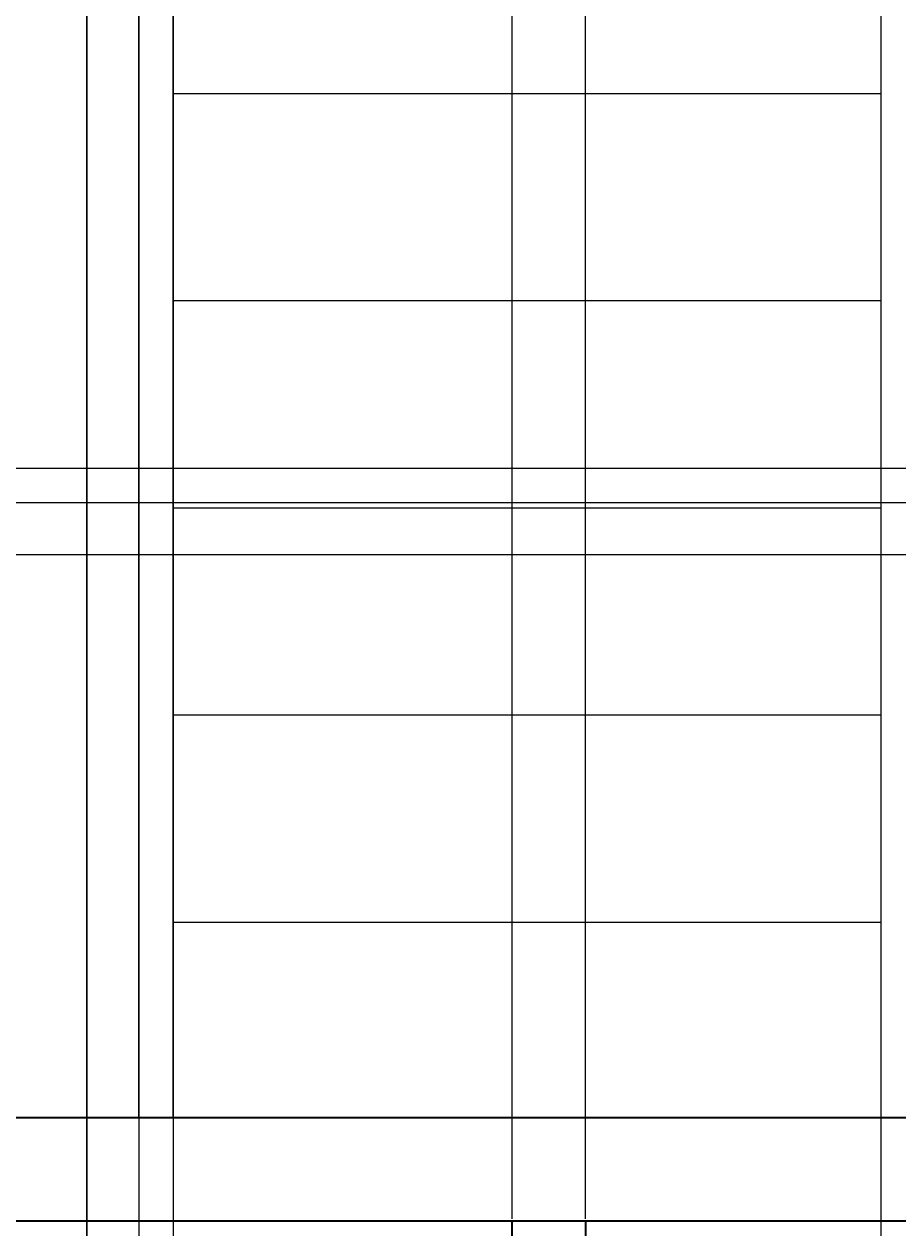
# Model space of a CAD drawing. Units: inches. Extents: x -6 to 289, y -8 to 323.
# Tile 67 of 107: x 186 to 212, y 159 to 194. Entities that reach past the tile are written whole.
import ezdxf

# ---------------------------------------------------------------- set-up
doc = ezdxf.new("R2010")
doc.units = ezdxf.units.IN
doc.header["$MEASUREMENT"] = 0
for name, color, linetype, lineweight in [('A-ANNO-DIMS', 2, 'Continuous', 18), ('A-ELEV', 7, 'Continuous', 35), ('A-ELEV-PATT', 8, 'Continuous', 13), ('A-GLAZ', 4, 'Continuous', 25)]:
    doc.layers.add(name, color=color, linetype=linetype, lineweight=lineweight)
doc.styles.get("Standard").update_dxf_attribs({"font": 'arial.ttf'})
doc.dimstyles.get("Standard").update_dxf_attribs({"dimtxt": 0.18, "dimasz": 0.18, "dimexe": 0.18, "dimexo": 0.0625, "dimgap": 0.09, "dimtad": 0, "dimtih": 1, "dimtoh": 1, "dimdec": 4, "dimzin": 0, "dimdsep": 46, "dimtxsty": 'Standard', "dimcen": 0.09, "dimadec": 0, "dimazin": 0, "dimtfac": 1, "dimtdec": 4, "dimtofl": 0, "dimtmove": 0, "dimatfit": 3, "dimfxl": 1, "dimtolj": 1, "dimtzin": 0, "dimarcsym": 0})

# ---------------------------------------------------------------- blocks, each defined once
blk = doc.blocks.new('*D24')
at = {"layer": 'A-ANNO-DIMS', "color": 0, "lineweight": -2, "transparency": 16777216}
for p, q in [((126.946, 178.654), (288.653, 178.654)), ((288.473, 178.474), (288.473, 159.153)), ((288.473, 139.469), (288.473, 158.789)), ((259.226, 139.289), (288.653, 139.289))]:
    blk.add_line(p, q, dxfattribs=at)
at = {"layer": 'A-ANNO-DIMS', "color": 0, "transparency": 16777216}
for points in [[(288.443, 178.474), (288.503, 178.474), (288.473, 178.654)], [(288.443, 139.469), (288.503, 139.469), (288.473, 139.289)]]:
    blk.add_solid(points, dxfattribs=at)
at = {"layer": 'Defpoints', "color": 0, "transparency": 16777216}
for p in [(126.883, 178.654), (288.473, 178.654), (259.164, 139.289)]:
    blk.add_point(p, dxfattribs=at)
at = {"layer": 'A-ANNO-DIMS', "color": 0, "transparency": 16777216, "insert": (288.473, 158.971), "char_height": 0.18, "attachment_point": 5}
blk.add_mtext('\\A1;39.365', dxfattribs=at)
blk = doc.blocks.new('*D25')
at = {"layer": 'A-ANNO-DIMS', "color": 0, "lineweight": -2, "transparency": 16777216}
for p, q in [((126.946, 226.654), (288.653, 226.654)), ((288.473, 226.474), (288.473, 202.836)), ((288.473, 178.834), (288.473, 202.472)), ((126.946, 178.654), (288.653, 178.654))]:
    blk.add_line(p, q, dxfattribs=at)
at = {"layer": 'A-ANNO-DIMS', "color": 0, "transparency": 16777216}
for points in [[(288.443, 226.474), (288.503, 226.474), (288.473, 226.654)], [(288.443, 178.834), (288.503, 178.834), (288.473, 178.654)]]:
    blk.add_solid(points, dxfattribs=at)
at = {"layer": 'Defpoints', "color": 0, "transparency": 16777216}
for p in [(126.883, 226.654), (288.473, 226.654), (126.883, 178.654)]:
    blk.add_point(p, dxfattribs=at)
at = {"layer": 'A-ANNO-DIMS', "color": 0, "transparency": 16777216, "insert": (288.473, 202.654), "char_height": 0.18, "attachment_point": 5}
blk.add_mtext('\\A1;48', dxfattribs=at)
blk = doc.blocks.new('*D35')
at = {"layer": 'A-ANNO-DIMS', "color": 0, "lineweight": -2, "transparency": 16777216}
for p, q in [((167.446, 180.154), (288.653, 180.154)), ((288.473, 179.974), (288.473, 179.586)), ((288.473, 178.834), (288.473, 179.222)), ((168.946, 178.654), (288.653, 178.654))]:
    blk.add_line(p, q, dxfattribs=at)
at = {"layer": 'A-ANNO-DIMS', "color": 0, "transparency": 16777216}
for points in [[(288.443, 179.974), (288.503, 179.974), (288.473, 180.154)], [(288.443, 178.834), (288.503, 178.834), (288.473, 178.654)]]:
    blk.add_solid(points, dxfattribs=at)
at = {"layer": 'Defpoints', "color": 0, "transparency": 16777216}
for p in [(167.383, 180.154), (288.473, 180.154), (168.883, 178.654)]:
    blk.add_point(p, dxfattribs=at)
at = {"layer": 'A-ANNO-DIMS', "color": 0, "transparency": 16777216, "insert": (288.473, 179.404), "char_height": 0.18, "attachment_point": 5}
blk.add_mtext('\\A1;1.5', dxfattribs=at)
blk = doc.blocks.new('*D36')
at = {"layer": 'A-ANNO-DIMS', "color": 0, "lineweight": -2, "transparency": 16777216}
for p, q in [((166.446, 181.154), (288.653, 181.154)), ((288.473, 180.974), (288.473, 180.834)), ((288.473, 180.334), (288.473, 180.474)), ((167.446, 180.154), (288.653, 180.154))]:
    blk.add_line(p, q, dxfattribs=at)
at = {"layer": 'A-ANNO-DIMS', "color": 0, "transparency": 16777216}
for points in [[(288.443, 180.974), (288.503, 180.974), (288.473, 181.154)], [(288.443, 180.334), (288.503, 180.334), (288.473, 180.154)]]:
    blk.add_solid(points, dxfattribs=at)
at = {"layer": 'Defpoints', "color": 0, "transparency": 16777216}
for p in [(166.383, 181.154), (288.473, 181.154), (167.383, 180.154)]:
    blk.add_point(p, dxfattribs=at)
at = {"layer": 'A-ANNO-DIMS', "color": 0, "transparency": 16777216, "insert": (288.473, 180.654), "char_height": 0.18, "attachment_point": 5}
blk.add_mtext('\\A1;1', dxfattribs=at)
blk = doc.blocks.new('*D37')
at = {"layer": 'A-ANNO-DIMS', "color": 0, "lineweight": -2, "transparency": 16777216}
for p, q in [((166.446, 224.154), (288.653, 224.154)), ((288.473, 223.974), (288.473, 202.836)), ((288.473, 181.334), (288.473, 202.472)), ((166.446, 181.154), (288.653, 181.154))]:
    blk.add_line(p, q, dxfattribs=at)
at = {"layer": 'A-ANNO-DIMS', "color": 0, "transparency": 16777216}
for points in [[(288.443, 223.974), (288.503, 223.974), (288.473, 224.154)], [(288.443, 181.334), (288.503, 181.334), (288.473, 181.154)]]:
    blk.add_solid(points, dxfattribs=at)
at = {"layer": 'Defpoints', "color": 0, "transparency": 16777216}
for p in [(166.383, 224.154), (288.473, 224.154), (166.383, 181.154)]:
    blk.add_point(p, dxfattribs=at)
at = {"layer": 'A-ANNO-DIMS', "color": 0, "transparency": 16777216, "insert": (288.473, 202.654), "char_height": 0.18, "attachment_point": 5}
blk.add_mtext('\\A1;43', dxfattribs=at)
blk = doc.blocks.new('*D40')
at = {"layer": 'A-ANNO-DIMS', "color": 0, "lineweight": -2, "transparency": 16777216}
for p, q in [((188.292, 226.826), (188.292, -8.391)), ((189.792, 225.326), (189.792, -8.391)), ((188.472, -8.211), (188.796, -8.211)), ((189.612, -8.211), (189.288, -8.211))]:
    blk.add_line(p, q, dxfattribs=at)
at = {"layer": 'A-ANNO-DIMS', "color": 0, "transparency": 16777216}
for points in [[(188.472, -8.181), (188.472, -8.241), (188.292, -8.211)], [(189.612, -8.181), (189.612, -8.241), (189.792, -8.211)]]:
    blk.add_solid(points, dxfattribs=at)
at = {"layer": 'Defpoints', "color": 0, "transparency": 16777216}
for p in [(188.292, 226.889), (189.792, 225.389), (189.792, -8.211)]:
    blk.add_point(p, dxfattribs=at)
at = {"layer": 'A-ANNO-DIMS', "color": 0, "transparency": 16777216, "insert": (189.042, -8.211), "char_height": 0.18, "attachment_point": 5}
blk.add_mtext('\\A1;1.5', dxfattribs=at)
blk = doc.blocks.new('*D41')
at = {"layer": 'A-ANNO-DIMS', "color": 0, "lineweight": -2, "transparency": 16777216}
for p, q in [((189.792, 225.326), (189.792, -8.391)), ((190.792, 224.326), (190.792, -8.391)), ((189.972, -8.211), (190.169, -8.211)), ((190.612, -8.211), (190.415, -8.211))]:
    blk.add_line(p, q, dxfattribs=at)
at = {"layer": 'A-ANNO-DIMS', "color": 0, "transparency": 16777216}
for points in [[(189.972, -8.181), (189.972, -8.241), (189.792, -8.211)], [(190.612, -8.181), (190.612, -8.241), (190.792, -8.211)]]:
    blk.add_solid(points, dxfattribs=at)
at = {"layer": 'Defpoints', "color": 0, "transparency": 16777216}
for p in [(189.792, 225.389), (190.792, 224.389), (190.792, -8.211)]:
    blk.add_point(p, dxfattribs=at)
at = {"layer": 'A-ANNO-DIMS', "color": 0, "transparency": 16777216, "insert": (190.292, -8.211), "char_height": 0.18, "attachment_point": 5}
blk.add_mtext('\\A1;1', dxfattribs=at)
blk = doc.blocks.new('*D42')
at = {"layer": 'A-ANNO-DIMS', "color": 0, "lineweight": -2, "transparency": 16777216}
for p, q in [((190.792, 224.326), (190.792, -8.391)), ((211.292, 224.326), (211.292, -8.391)), ((190.972, -8.211), (200.716, -8.211)), ((211.112, -8.211), (201.368, -8.211))]:
    blk.add_line(p, q, dxfattribs=at)
at = {"layer": 'A-ANNO-DIMS', "color": 0, "transparency": 16777216}
for points in [[(190.972, -8.181), (190.972, -8.241), (190.792, -8.211)], [(211.112, -8.181), (211.112, -8.241), (211.292, -8.211)]]:
    blk.add_solid(points, dxfattribs=at)
at = {"layer": 'Defpoints', "color": 0, "transparency": 16777216}
for p in [(190.792, 224.389), (211.292, 224.389), (211.292, -8.211)]:
    blk.add_point(p, dxfattribs=at)
at = {"layer": 'A-ANNO-DIMS', "color": 0, "transparency": 16777216, "insert": (201.042, -8.211), "char_height": 0.18, "attachment_point": 5}
blk.add_mtext('\\A1;20.5', dxfattribs=at)
blk = doc.blocks.new('*D43')
at = {"layer": 'A-ANNO-DIMS', "color": 0, "lineweight": -2, "transparency": 16777216}
for p, q in [((211.292, 224.326), (211.292, -8.391)), ((212.292, 224.326), (212.292, -8.391)), ((211.472, -8.211), (211.669, -8.211)), ((212.112, -8.211), (211.915, -8.211))]:
    blk.add_line(p, q, dxfattribs=at)
at = {"layer": 'A-ANNO-DIMS', "color": 0, "transparency": 16777216}
for points in [[(211.472, -8.181), (211.472, -8.241), (211.292, -8.211)], [(212.112, -8.181), (212.112, -8.241), (212.292, -8.211)]]:
    blk.add_solid(points, dxfattribs=at)
at = {"layer": 'Defpoints', "color": 0, "transparency": 16777216}
for p in [(211.292, 224.389), (212.292, 224.389), (212.292, -8.211)]:
    blk.add_point(p, dxfattribs=at)
at = {"layer": 'A-ANNO-DIMS', "color": 0, "transparency": 16777216, "insert": (211.792, -8.211), "char_height": 0.18, "attachment_point": 5}
blk.add_mtext('\\A1;1', dxfattribs=at)
blk = doc.blocks.new('*D79')
at = {"layer": 'A-ANNO-DIMS', "color": 0, "lineweight": -2, "transparency": 16777216}
for p, q in [((171.296, 118.033), (171.296, 322.969)), ((188.292, 116.842), (188.292, 322.969)), ((171.476, 322.789), (179.339, 322.789)), ((188.112, 322.789), (180.249, 322.789))]:
    blk.add_line(p, q, dxfattribs=at)
at = {"layer": 'A-ANNO-DIMS', "color": 0, "transparency": 16777216}
for points in [[(171.476, 322.819), (171.476, 322.759), (171.296, 322.789)], [(188.112, 322.819), (188.112, 322.759), (188.292, 322.789)]]:
    blk.add_solid(points, dxfattribs=at)
at = {"layer": 'Defpoints', "color": 0, "transparency": 16777216}
for p in [(188.292, 322.789), (171.296, 117.971), (188.292, 116.779)]:
    blk.add_point(p, dxfattribs=at)
at = {"layer": 'A-ANNO-DIMS', "color": 0, "transparency": 16777216, "insert": (179.794, 322.789), "char_height": 0.18, "attachment_point": 5}
blk.add_mtext('\\A1;16.996', dxfattribs=at)
blk = doc.blocks.new('*D80')
at = {"layer": 'A-ANNO-DIMS', "color": 0, "lineweight": -2, "transparency": 16777216}
for p, q in [((188.292, 116.842), (188.292, 322.969)), ((230.292, 116.842), (230.292, 322.969)), ((188.472, 322.789), (209.07, 322.789)), ((230.112, 322.789), (209.513, 322.789))]:
    blk.add_line(p, q, dxfattribs=at)
at = {"layer": 'A-ANNO-DIMS', "color": 0, "transparency": 16777216}
for points in [[(188.472, 322.819), (188.472, 322.759), (188.292, 322.789)], [(230.112, 322.819), (230.112, 322.759), (230.292, 322.789)]]:
    blk.add_solid(points, dxfattribs=at)
at = {"layer": 'Defpoints', "color": 0, "transparency": 16777216}
for p in [(230.292, 322.789), (188.292, 116.779), (230.292, 116.779)]:
    blk.add_point(p, dxfattribs=at)
at = {"layer": 'A-ANNO-DIMS', "color": 0, "transparency": 16777216, "insert": (209.292, 322.789), "char_height": 0.18, "attachment_point": 5}
blk.add_mtext('\\A1;42', dxfattribs=at)
blk = doc.blocks.new('*D96')
at = {"layer": 'A-ANNO-DIMS', "color": 0, "lineweight": -2, "transparency": 16777216}
for p, q in [((164.004, 159.411), (164.004, 322.969)), ((200.616, 159.411), (200.616, 322.969)), ((164.184, 322.789), (181.934, 322.789)), ((200.436, 322.789), (182.686, 322.789))]:
    blk.add_line(p, q, dxfattribs=at)
at = {"layer": 'A-ANNO-DIMS', "color": 0, "transparency": 16777216}
for points in [[(164.184, 322.819), (164.184, 322.759), (164.004, 322.789)], [(200.436, 322.819), (200.436, 322.759), (200.616, 322.789)]]:
    blk.add_solid(points, dxfattribs=at)
at = {"layer": 'Defpoints', "color": 0, "transparency": 16777216}
for p in [(200.616, 322.789), (164.004, 159.348), (200.616, 159.348)]:
    blk.add_point(p, dxfattribs=at)
at = {"layer": 'A-ANNO-DIMS', "color": 0, "transparency": 16777216, "insert": (182.31, 322.789), "char_height": 0.18, "attachment_point": 5}
blk.add_mtext('\\A1;36.61', dxfattribs=at)
blk = doc.blocks.new('*D97')
at = {"layer": 'A-ANNO-DIMS', "color": 0, "lineweight": -2, "transparency": 16777216}
for p, q in [((200.616, 159.411), (200.616, 322.969)), ((202.741, 159.411), (202.741, 322.969)), ((200.796, 322.789), (201.283, 322.789)), ((202.561, 322.789), (202.075, 322.789))]:
    blk.add_line(p, q, dxfattribs=at)
at = {"layer": 'A-ANNO-DIMS', "color": 0, "transparency": 16777216}
for points in [[(200.796, 322.819), (200.796, 322.759), (200.616, 322.789)], [(202.561, 322.819), (202.561, 322.759), (202.741, 322.789)]]:
    blk.add_solid(points, dxfattribs=at)
at = {"layer": 'Defpoints', "color": 0, "transparency": 16777216}
for p in [(202.741, 322.789), (200.616, 159.348), (202.741, 159.348)]:
    blk.add_point(p, dxfattribs=at)
at = {"layer": 'A-ANNO-DIMS', "color": 0, "transparency": 16777216, "insert": (201.679, 322.789), "char_height": 0.18, "attachment_point": 5}
blk.add_mtext('\\A1;2.125', dxfattribs=at)
blk = doc.blocks.new('*D98')
at = {"layer": 'A-ANNO-DIMS', "color": 0, "lineweight": -2, "transparency": 16777216}
for p, q in [((202.741, 159.411), (202.741, 322.969)), ((244.164, 159.411), (244.164, 322.969)), ((202.921, 322.789), (223.056, 322.789)), ((243.984, 322.789), (223.849, 322.789))]:
    blk.add_line(p, q, dxfattribs=at)
at = {"layer": 'A-ANNO-DIMS', "color": 0, "transparency": 16777216}
for points in [[(202.921, 322.819), (202.921, 322.759), (202.741, 322.789)], [(243.984, 322.819), (243.984, 322.759), (244.164, 322.789)]]:
    blk.add_solid(points, dxfattribs=at)
at = {"layer": 'Defpoints', "color": 0, "transparency": 16777216}
for p in [(244.164, 322.789), (202.741, 159.348), (244.164, 159.348)]:
    blk.add_point(p, dxfattribs=at)
at = {"layer": 'A-ANNO-DIMS', "color": 0, "transparency": 16777216, "insert": (223.452, 322.789), "char_height": 0.18, "attachment_point": 5}
blk.add_mtext('\\A1;41.42', dxfattribs=at)

msp = doc.modelspace()

# ---------------------------------------------------------------- hatches: boundary and pattern name
at = {"layer": 'A-ELEV-PATT'}
h = msp.add_hatch(dxfattribs=at)
h.set_pattern_fill('_USER', color=256, scale=6, pattern_type=0)
h.set_pattern_definition([(0, (0, 0), (0, 6), [])])
h.paths.add_polyline_path([(184.1244, 48.0851), (124.008, 48.0851), (124.008, 10.2888), (184.1244, 10.2888)])
h.paths.add_polyline_path([(244.2408, 48.0851), (186.3604, 48.0851), (186.3604, 10.2888), (244.2408, 10.2888)])
h.paths.add_polyline_path([(208.2918, 114.2795), (190.7918, 114.2795), (190.7918, 71.2795), (208.2918, 71.2795)])
h.paths.add_polyline_path([(227.7918, 114.2795), (209.2918, 114.2795), (209.2918, 71.2795), (227.7918, 71.2795)])
h.paths.add_polyline_path([(211.2918, 224.3887), (190.7918, 224.3887), (190.7918, 162.3484), (211.2918, 162.3484)])
h.paths.add_polyline_path([(233.7918, 224.3887), (212.2918, 224.3887), (212.2918, 162.3484), (233.7918, 162.3484)])
h.paths.add_polyline_path([(166.3835, 224.154), (147.8835, 224.154), (147.8835, 181.154), (166.3835, 181.154)])
h.paths.add_polyline_path([(146.8835, 224.154), (129.3835, 224.154), (129.3835, 181.154), (146.8835, 181.154)])

# ---------------------------------------------------------------- linework, layer by layer
at = {"layer": 'A-ELEV'}
for points in [[(247.1638, 139.2888), (115.1638, 139.2888), (115.1638, 162.3484), (247.1638, 162.3484)], [(244.1638, 142.2888), (118.1638, 142.2888), (118.1638, 159.3484), (244.1638, 159.3484)], [(200.6162, 159.3484), (202.741, 159.3484), (202.741, 142.2888), (200.6162, 142.2888)]]:
    msp.add_lwpolyline(points, close=True, dxfattribs=at)
at = {"layer": 'A-GLAZ'}
msp.add_line((189.7918, 162.3484), (189.7918, 225.3887), dxfattribs=at)
for points in [[(188.2918, 162.3484), (188.2918, 226.8887), (236.2918, 226.8887), (236.2918, 162.3484)], [(190.7918, 162.3484), (190.7918, 224.3887), (211.2918, 224.3887)], [(211.2918, 224.3887), (211.2918, 162.3484)]]:
    msp.add_lwpolyline(points, dxfattribs=at)

# ---------------------------------------------------------------- dimensions: what is measured, and where the dimension line sits
at = {"layer": 'A-ANNO-DIMS'}
for base, p1, p2, override, picture, middle in [((200.6162, 322.7888), (164.0039, 159.3484), (200.6162, 159.3484), {"dimdec": 2, "dimlfac": 1, "dimrnd": 0, "dimzin": 0, "dimdsep": 46, "dimlunit": 2}, '*D96', (182.3101, 322.7888)), ((188.2918, 322.7888), (171.296, 117.9706), (188.2918, 116.7795), {"dimdec": 3, "dimlfac": 1, "dimrnd": 0, "dimzin": 0, "dimdsep": 46, "dimlunit": 2}, '*D79', (179.7939, 322.7888)), ((230.2918, 322.7888), (188.2918, 116.7795), (230.2918, 116.7795), {"dimdec": 0, "dimlfac": 1, "dimrnd": 0, "dimzin": 0, "dimdsep": 46, "dimlunit": 2}, '*D80', (209.2918, 322.7888)), ((202.741, 322.7888), (200.6162, 159.3484), (202.741, 159.3484), {"dimdec": 3, "dimlfac": 1, "dimrnd": 0, "dimzin": 0, "dimdsep": 46, "dimlunit": 2}, '*D97', (201.6786, 322.7888)), ((244.1638, 322.7888), (202.741, 159.3484), (244.1638, 159.3484), {"dimdec": 2, "dimlfac": 1, "dimrnd": 0, "dimzin": 0, "dimdsep": 46, "dimlunit": 2}, '*D98', (223.4524, 322.7888)), ((189.7918, -8.2112), (188.2918, 226.8887), (189.7918, 225.3887), {"dimdec": 1, "dimlfac": 1, "dimrnd": 0, "dimzin": 0, "dimdsep": 46, "dimlunit": 2}, '*D40', (189.0418, -8.2112)), ((190.7918, -8.2112), (189.7918, 225.3887), (190.7918, 224.3887), {"dimdec": 0, "dimlfac": 1, "dimrnd": 0, "dimzin": 0, "dimdsep": 46, "dimlunit": 2}, '*D41', (190.2918, -8.2112)), ((211.2918, -8.2112), (190.7918, 224.3887), (211.2918, 224.3887), {"dimdec": 1, "dimlfac": 1, "dimrnd": 0, "dimzin": 0, "dimdsep": 46, "dimlunit": 2}, '*D42', (201.0418, -8.2112)), ((212.2918, -8.2112), (211.2918, 224.3887), (212.2918, 224.3887), {"dimdec": 0, "dimlfac": 1, "dimrnd": 0, "dimzin": 0, "dimdsep": 46, "dimlunit": 2}, '*D43', (211.7918, -8.2112))]:
    dim = msp.add_linear_dim(base=base, p1=p1, p2=p2, dimstyle='Standard', override=override, dxfattribs=at)
    dim.commit()
    dim.dimension.update_dxf_attribs({"geometry": picture, "text_midpoint": middle})
for base, p1, p2, override, picture, middle in [((288.4733, 226.654), (126.8835, 178.654), (126.8835, 226.654), {"dimdec": 0, "dimlfac": 1, "dimrnd": 0, "dimzin": 0, "dimdsep": 46, "dimlunit": 2}, '*D25', (288.4733, 202.654)), ((288.4733, 224.154), (166.3835, 181.154), (166.3835, 224.154), {"dimdec": 0, "dimlfac": 1, "dimrnd": 0, "dimzin": 0, "dimdsep": 46, "dimlunit": 2}, '*D37', (288.4733, 202.654)), ((288.4733, 181.154), (167.3835, 180.154), (166.3835, 181.154), {"dimdec": 0, "dimlfac": 1, "dimrnd": 0, "dimzin": 0, "dimdsep": 46, "dimlunit": 2}, '*D36', (288.4733, 180.654)), ((288.4733, 180.154), (168.8835, 178.654), (167.3835, 180.154), {"dimdec": 1, "dimlfac": 1, "dimrnd": 0, "dimzin": 0, "dimdsep": 46, "dimlunit": 2}, '*D35', (288.4733, 179.404)), ((288.4733, 178.654), (259.1638, 139.2888), (126.8835, 178.654), {"dimdec": 3, "dimlfac": 1, "dimrnd": 0, "dimzin": 0, "dimdsep": 46, "dimlunit": 2}, '*D24', (288.4733, 158.9714))]:
    dim = msp.add_linear_dim(base=base, p1=p1, p2=p2, angle=90, dimstyle='Standard', override=override, dxfattribs=at)
    dim.commit()
    dim.dimension.update_dxf_attribs({"geometry": picture, "text_midpoint": middle})

doc.saveas('drawing.dxf')
